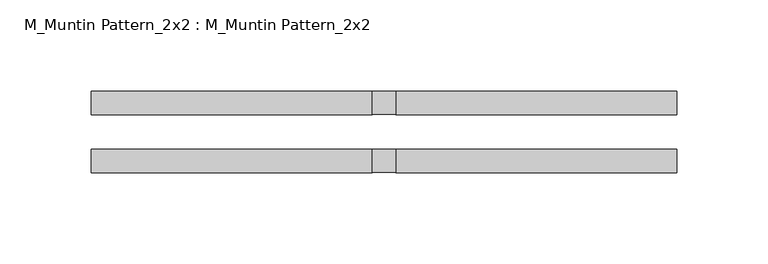
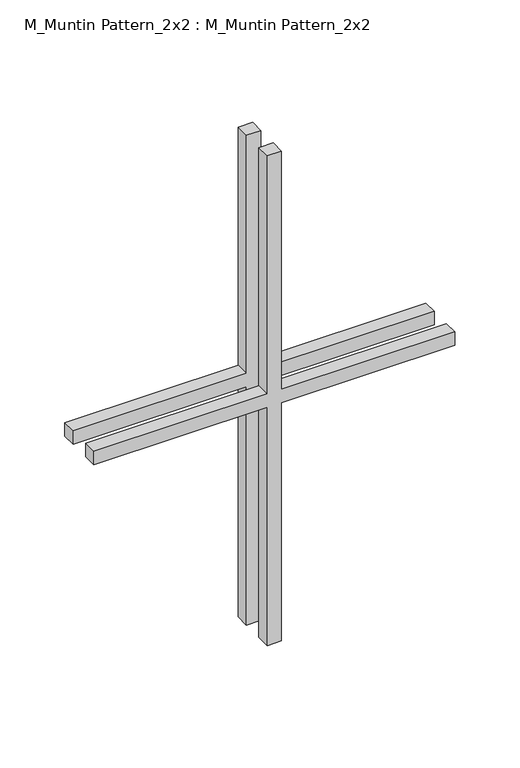
"""IFC4 building model written with IfcOpenShell, lengths in millimetres: proxy geometry, M_Muntin Pattern_2x2 : M_Muntin Pattern_2x2."""

from ifc_helpers import new_model, si_unit, frame, origin, place, context, project, spatial, polyline, outline, extrude, source, transform, mapped, element, save


def m_muntin_pattern_2x2_m_muntin_pattern_2x2_8c7fd3cb(model_context):
    return source(origin(), model_context, "Body", "SweptSolid", [
        extrude(outline(polyline([(236.5, -6.35), (236.5, -160.3375), (223.8, -160.3375), (223.8, -6.35), (0.0, -6.35), (0.0, 6.35), (223.8, 6.35), (223.8, 160.3375), (236.5, 160.3375), (236.5, 6.35), (460.3, 6.35), (460.3, -6.35), (236.5, -6.35)])), frame((0.0, -22.225, 0.0), z_axis=(0.0, 1.0, 0.0), x_axis=(0.0, 0.0, 1.0)), (0.0, 0.0, 1.0), 12.7),
        extrude(outline(polyline([(236.5, -6.35), (236.5, -160.3375), (223.8, -160.3375), (223.8, -6.35), (0.0, -6.35), (0.0, 6.35), (223.8, 6.35), (223.8, 160.3375), (236.5, 160.3375), (236.5, 6.35), (460.3, 6.35), (460.3, -6.35), (236.5, -6.35)])), frame((0.0, 9.525, 0.0), z_axis=(0.0, 1.0, 0.0), x_axis=(0.0, 0.0, 1.0)), (0.0, 0.0, 1.0), 12.7),
    ])


if __name__ == "__main__":
    model = new_model("IFC4")
    model_context = context("Model", 3, world=origin())
    ifc_project = project(units=[si_unit("LENGTHUNIT", "METRE", prefix="MILLI")], contexts=[model_context])
    site = spatial("IfcSite", under=ifc_project)
    building = spatial("IfcBuilding", under=site)
    placement = place(None, origin())
    m_muntin_pattern_2x2_m_muntin_pattern_2x2_shape = m_muntin_pattern_2x2_m_muntin_pattern_2x2_8c7fd3cb(model_context)
    element("IfcBuildingElementProxy", 1, Name="M_Muntin Pattern_2x2 : M_Muntin Pattern_2x2", ObjectType="M_Muntin Pattern_2x2 : M_Muntin Pattern_2x2", at=placement, inside=building, context=model_context, shape_type="MappedRepresentation", body=[
        mapped(m_muntin_pattern_2x2_m_muntin_pattern_2x2_shape, transform((0.0, 0.0, 0.0), x_axis=(1.0, 0.0, 0.0), y_axis=(0.0, 1.0, 0.0), z_axis=(0.0, 0.0, 1.0))),
    ])
    save(model, "model.ifc")

# Revit data of these elements
# Type "M_Muntin Pattern_2x2 : M_Muntin Pattern_2x2"
#   Width [instance default] = 3' - 11.24409"
#   Thickness = 0' - 0 1/2"
#   Height [instance default] = 3' - 11.24409"
#   Distance = 0' - 0 3/4"
#   Interior Material [instance default] = none
#   Exterior Material [instance default] = none
#   Default Elevation = 0
# Element 1 (IfcBuildingElementProxy, "M_Muntin Pattern_2x2 : M_Muntin Pattern_2x2")
#   Width = 1' - 0 5/8"
#   Height = 1' - 6.12205"
#   Interior Material = Wood - Stained
#   Exterior Material = Clad - White
#   Materials on its faces: "Clad - White", "Wood - Stained"
# Materials
#   "Clad - White": class "Wood", colour RGB 242 242 238, transparency 0, Cost = 0
#   "Wood - Stained": class "Wood", colour RGB 224 178 126, transparency 0, Cost = 0
